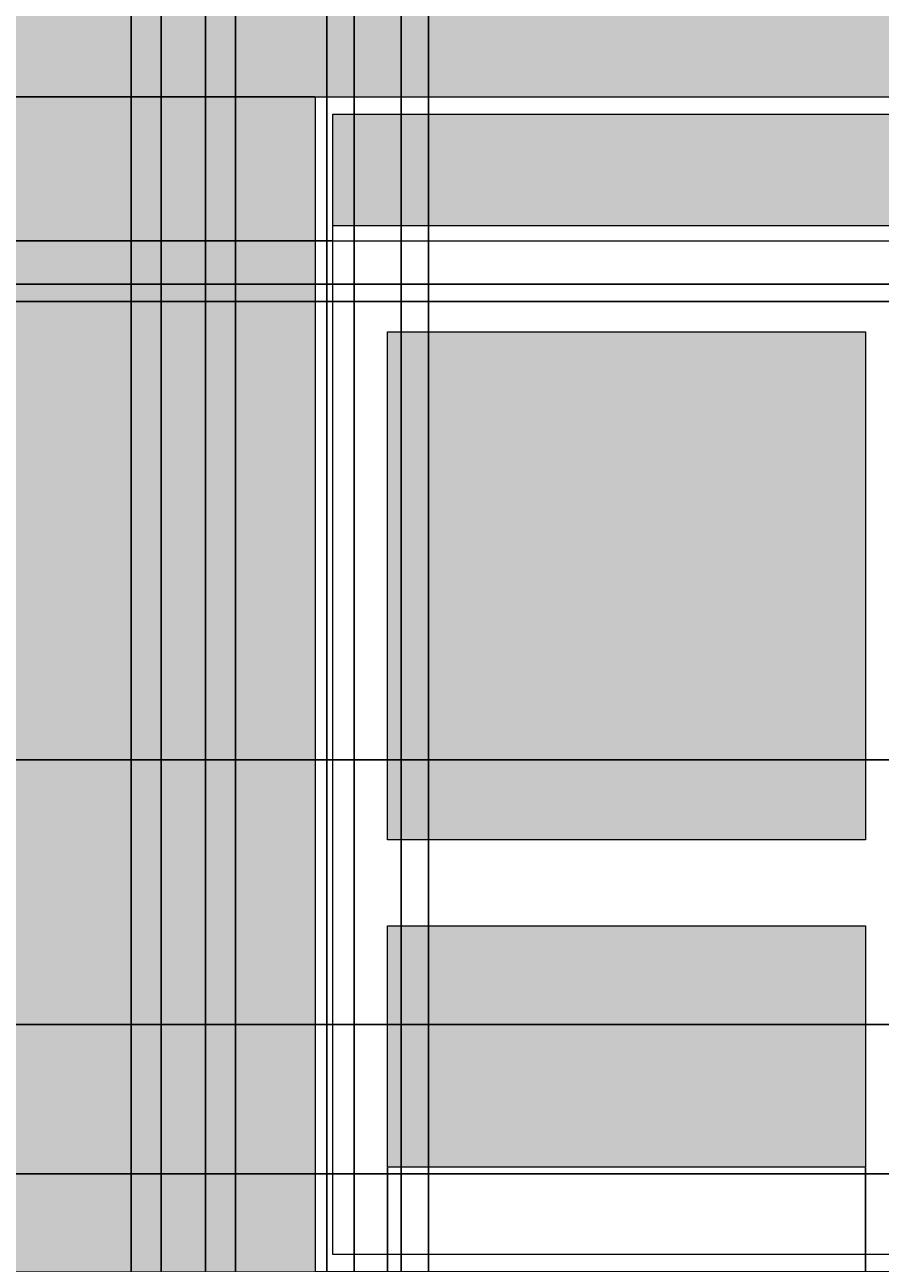
# Model space of a CAD drawing. Units: inches. Extents: x 36 to 594, y 79 to 831.
# Tile 5 of 30: x 221 to 319, y 152 to 294. Entities that reach past the tile are written whole.
import ezdxf

# ---------------------------------------------------------------- set-up
doc = ezdxf.new("R2010")
doc.units = ezdxf.units.IN
doc.header["$MEASUREMENT"] = 0
for name, color, linetype, lineweight in [('A-ANNO-DIMS', 2, 'Continuous', 18), ('A-DOOR', 3, 'Continuous', 18), ('A-ELEV-PATT', 8, 'Continuous', 13)]:
    doc.layers.add(name, color=color, linetype=linetype, lineweight=lineweight)
doc.styles.get("Standard").update_dxf_attribs({"font": 'arial.ttf'})
doc.dimstyles.get("Standard").update_dxf_attribs({"dimtxt": 0.8125, "dimasz": 0.18, "dimexe": 0.18, "dimexo": 0.0625, "dimgap": 0.09, "dimtad": 0, "dimtih": 1, "dimtoh": 1, "dimdec": 4, "dimzin": 0, "dimdsep": 46, "dimlunit": 4, "dimtxsty": 'Standard', "dimcen": 0.09, "dimadec": 0, "dimazin": 0, "dimtfac": 1, "dimtdec": 4, "dimtofl": 0, "dimtmove": 0, "dimatfit": 3, "dimfxl": 1, "dimtolj": 1, "dimtzin": 0, "dimarcsym": 0})

# ---------------------------------------------------------------- blocks, each defined once
blk = doc.blocks.new('*D28')
at = {"layer": 'A-ANNO-DIMS', "color": 0, "lineweight": -2, "transparency": 16777216}
for p, q in [((269.3, 796.05), (37.49, 796.05)), ((37.67, 795.87), (37.67, 455.63)), ((37.67, 114.39), (37.67, 454.62)), ((94.8, 114.21), (37.49, 114.21))]:
    blk.add_line(p, q, dxfattribs=at)
at = {"layer": 'A-ANNO-DIMS', "color": 0, "transparency": 16777216}
for points in [[(37.64, 795.87), (37.7, 795.87), (37.67, 796.05)], [(37.64, 114.39), (37.7, 114.39), (37.67, 114.21)]]:
    blk.add_solid(points, dxfattribs=at)
at = {"layer": 'Defpoints', "color": 0, "transparency": 16777216}
for p in [(37.67, 796.05), (269.36, 796.05), (94.87, 114.21)]:
    blk.add_point(p, dxfattribs=at)
at = {"layer": 'A-ANNO-DIMS', "color": 0, "transparency": 16777216, "insert": (37.67, 455.13), "char_height": 0.812, "attachment_point": 5}
blk.add_mtext('\\A1;681.8', dxfattribs=at)
blk = doc.blocks.new('*D74')
at = {"layer": 'A-ANNO-DIMS', "color": 0, "lineweight": -2, "transparency": 16777216}
for p, q in [((217.09, 179.42), (592.85, 179.42)), ((592.67, 179.24), (592.67, 171.32)), ((592.67, 162.39), (592.67, 170.31)), ((217.09, 162.21), (592.85, 162.21))]:
    blk.add_line(p, q, dxfattribs=at)
at = {"layer": 'A-ANNO-DIMS', "color": 0, "transparency": 16777216}
for points in [[(592.64, 179.24), (592.7, 179.24), (592.67, 179.42)], [(592.64, 162.39), (592.7, 162.39), (592.67, 162.21)]]:
    blk.add_solid(points, dxfattribs=at)
at = {"layer": 'Defpoints', "color": 0, "transparency": 16777216}
for p in [(217.03, 179.42), (592.67, 179.42), (217.03, 162.21)]:
    blk.add_point(p, dxfattribs=at)
at = {"layer": 'A-ANNO-DIMS', "color": 0, "transparency": 16777216, "insert": (592.67, 170.82), "char_height": 0.812, "attachment_point": 5}
blk.add_mtext('\\A1;17.207', dxfattribs=at)
blk = doc.blocks.new('*D75')
at = {"layer": 'A-ANNO-DIMS', "color": 0, "lineweight": -2, "transparency": 16777216}
for p, q in [((215.09, 262.62), (592.85, 262.62)), ((592.67, 262.44), (592.67, 221.53)), ((592.67, 179.6), (592.67, 220.52)), ((217.09, 179.42), (592.85, 179.42))]:
    blk.add_line(p, q, dxfattribs=at)
at = {"layer": 'A-ANNO-DIMS', "color": 0, "transparency": 16777216}
for points in [[(592.64, 262.44), (592.7, 262.44), (592.67, 262.62)], [(592.64, 179.6), (592.7, 179.6), (592.67, 179.42)]]:
    blk.add_solid(points, dxfattribs=at)
at = {"layer": 'Defpoints', "color": 0, "transparency": 16777216}
for p in [(215.03, 262.62), (592.67, 262.62), (217.03, 179.42)]:
    blk.add_point(p, dxfattribs=at)
at = {"layer": 'A-ANNO-DIMS', "color": 0, "transparency": 16777216, "insert": (592.67, 221.02), "char_height": 0.812, "attachment_point": 5}
blk.add_mtext('\\A1;83.2', dxfattribs=at)
blk = doc.blocks.new('*D76')
at = {"layer": 'A-ANNO-DIMS', "color": 0, "lineweight": -2, "transparency": 16777216}
for p, q in [((217.09, 264.62), (592.85, 264.62)), ((592.67, 264.44), (592.67, 264.12)), ((215.09, 262.62), (592.85, 262.62)), ((592.67, 262.8), (592.67, 263.12))]:
    blk.add_line(p, q, dxfattribs=at)
at = {"layer": 'A-ANNO-DIMS', "color": 0, "transparency": 16777216}
for points in [[(592.64, 264.44), (592.7, 264.44), (592.67, 264.62)], [(592.64, 262.8), (592.7, 262.8), (592.67, 262.62)]]:
    blk.add_solid(points, dxfattribs=at)
at = {"layer": 'Defpoints', "color": 0, "transparency": 16777216}
for p in [(217.03, 264.62), (592.67, 264.62), (215.03, 262.62)]:
    blk.add_point(p, dxfattribs=at)
at = {"layer": 'A-ANNO-DIMS', "color": 0, "transparency": 16777216, "insert": (592.67, 263.62), "char_height": 0.812, "attachment_point": 5}
blk.add_mtext('\\A1;2', dxfattribs=at)
blk = doc.blocks.new('*D77')
at = {"layer": 'A-ANNO-DIMS', "color": 0, "lineweight": -2, "transparency": 16777216}
for p, q in [((151.64, 209.88), (592.85, 209.88)), ((592.67, 209.7), (592.67, 186.55)), ((592.67, 162.39), (592.67, 185.54)), ((156.47, 162.21), (592.85, 162.21))]:
    blk.add_line(p, q, dxfattribs=at)
at = {"layer": 'A-ANNO-DIMS', "color": 0, "transparency": 16777216}
for points in [[(592.64, 209.7), (592.7, 209.7), (592.67, 209.88)], [(592.64, 162.39), (592.7, 162.39), (592.67, 162.21)]]:
    blk.add_solid(points, dxfattribs=at)
at = {"layer": 'Defpoints', "color": 0, "transparency": 16777216}
for p in [(151.58, 209.88), (156.41, 162.21), (592.67, 162.21)]:
    blk.add_point(p, dxfattribs=at)
at = {"layer": 'A-ANNO-DIMS', "color": 0, "transparency": 16777216, "insert": (592.67, 186.05), "char_height": 0.812, "attachment_point": 5}
blk.add_mtext('\\A1;47.67', dxfattribs=at)
blk = doc.blocks.new('*D78')
at = {"layer": 'A-ANNO-DIMS', "color": 0, "lineweight": -2, "transparency": 16777216}
for p, q in [((262.32, 162.93), (262.32, 79.53)), ((254.03, 150.87), (254.03, 79.53)), ((254.21, 79.71), (256.71, 79.71)), ((262.14, 79.71), (259.64, 79.71))]:
    blk.add_line(p, q, dxfattribs=at)
at = {"layer": 'A-ANNO-DIMS', "color": 0, "transparency": 16777216}
for points in [[(254.21, 79.74), (254.21, 79.68), (254.03, 79.71)], [(262.14, 79.74), (262.14, 79.68), (262.32, 79.71)]]:
    blk.add_solid(points, dxfattribs=at)
at = {"layer": 'Defpoints', "color": 0, "transparency": 16777216}
for p in [(262.32, 162.99), (254.03, 150.93), (262.32, 79.71)]:
    blk.add_point(p, dxfattribs=at)
at = {"layer": 'A-ANNO-DIMS', "color": 0, "transparency": 16777216, "insert": (258.17, 79.71), "char_height": 0.812, "attachment_point": 5}
blk.add_mtext('\\A1;8.288', dxfattribs=at)
blk = doc.blocks.new('*D79')
at = {"layer": 'A-ANNO-DIMS', "color": 0, "lineweight": -2, "transparency": 16777216}
for p, q in [((262.32, 162.93), (262.32, 79.53)), ((317.35, 162.93), (317.35, 79.53)), ((262.5, 79.71), (288.38, 79.71)), ((317.17, 79.71), (291.29, 79.71))]:
    blk.add_line(p, q, dxfattribs=at)
at = {"layer": 'A-ANNO-DIMS', "color": 0, "transparency": 16777216}
for points in [[(262.5, 79.74), (262.5, 79.68), (262.32, 79.71)], [(317.17, 79.74), (317.17, 79.68), (317.35, 79.71)]]:
    blk.add_solid(points, dxfattribs=at)
at = {"layer": 'Defpoints', "color": 0, "transparency": 16777216}
for p in [(262.32, 162.99), (317.35, 162.99), (317.35, 79.71)]:
    blk.add_point(p, dxfattribs=at)
at = {"layer": 'A-ANNO-DIMS', "color": 0, "transparency": 16777216, "insert": (289.84, 79.71), "char_height": 0.812, "attachment_point": 5}
blk.add_mtext('\\A1;55.04', dxfattribs=at)
blk = doc.blocks.new('*D80')
at = {"layer": 'A-ANNO-DIMS', "color": 0, "lineweight": -2, "transparency": 16777216}
for p, q in [((317.35, 162.93), (317.35, 79.53)), ((327.79, 152.87), (327.79, 79.53)), ((317.53, 79.71), (320.83, 79.71)), ((327.61, 79.71), (324.31, 79.71))]:
    blk.add_line(p, q, dxfattribs=at)
at = {"layer": 'A-ANNO-DIMS', "color": 0, "transparency": 16777216}
for points in [[(317.53, 79.74), (317.53, 79.68), (317.35, 79.71)], [(327.61, 79.74), (327.61, 79.68), (327.79, 79.71)]]:
    blk.add_solid(points, dxfattribs=at)
at = {"layer": 'Defpoints', "color": 0, "transparency": 16777216}
for p in [(317.35, 162.99), (327.79, 152.93), (327.79, 79.71)]:
    blk.add_point(p, dxfattribs=at)
at = {"layer": 'A-ANNO-DIMS', "color": 0, "transparency": 16777216, "insert": (322.57, 79.71), "char_height": 0.812, "attachment_point": 5}
blk.add_mtext('\\A1;10.436', dxfattribs=at)
blk = doc.blocks.new('*D90')
at = {"layer": 'A-ANNO-DIMS', "color": 0, "lineweight": -2, "transparency": 16777216}
for p, q in [((255.97, 269.61), (37.49, 269.61)), ((37.67, 269.43), (37.67, 210.78)), ((37.67, 151.11), (37.67, 209.77)), ((253.97, 150.93), (37.49, 150.93))]:
    blk.add_line(p, q, dxfattribs=at)
at = {"layer": 'A-ANNO-DIMS', "color": 0, "transparency": 16777216}
for points in [[(37.64, 269.43), (37.7, 269.43), (37.67, 269.61)], [(37.64, 151.11), (37.7, 151.11), (37.67, 150.93)]]:
    blk.add_solid(points, dxfattribs=at)
at = {"layer": 'Defpoints', "color": 0, "transparency": 16777216}
for p in [(37.67, 269.61), (256.03, 269.61), (254.03, 150.93)]:
    blk.add_point(p, dxfattribs=at)
at = {"layer": 'A-ANNO-DIMS', "color": 0, "transparency": 16777216, "insert": (37.67, 210.27), "char_height": 0.812, "attachment_point": 5}
blk.add_mtext('\\A1;118.67', dxfattribs=at)
blk = doc.blocks.new('*D91')
at = {"layer": 'A-ANNO-DIMS', "color": 0, "lineweight": -2, "transparency": 16777216}
for p, q in [((253.97, 286.18), (37.49, 286.18)), ((37.67, 286), (37.67, 278.4)), ((37.67, 269.79), (37.67, 277.39)), ((255.97, 269.61), (37.49, 269.61))]:
    blk.add_line(p, q, dxfattribs=at)
at = {"layer": 'A-ANNO-DIMS', "color": 0, "transparency": 16777216}
for points in [[(37.64, 286), (37.7, 286), (37.67, 286.18)], [(37.64, 269.79), (37.7, 269.79), (37.67, 269.61)]]:
    blk.add_solid(points, dxfattribs=at)
at = {"layer": 'Defpoints', "color": 0, "transparency": 16777216}
for p in [(37.67, 286.18), (254.03, 286.18), (256.03, 269.61)]:
    blk.add_point(p, dxfattribs=at)
at = {"layer": 'A-ANNO-DIMS', "color": 0, "transparency": 16777216, "insert": (37.67, 277.89), "char_height": 0.812, "attachment_point": 5}
blk.add_mtext('\\A1;16.572', dxfattribs=at)
blk = doc.blocks.new('*D96')
at = {"layer": 'A-ANNO-DIMS', "color": 0, "lineweight": -2, "transparency": 16777216}
for p, q in [((236.29, 484.36), (236.29, 79.53)), ((232.82, 475.35), (232.82, 79.53)), ((233, 79.71), (233.41, 79.71)), ((236.11, 79.71), (235.7, 79.71))]:
    blk.add_line(p, q, dxfattribs=at)
at = {"layer": 'A-ANNO-DIMS', "color": 0, "transparency": 16777216}
for points in [[(233, 79.74), (233, 79.68), (232.82, 79.71)], [(236.11, 79.74), (236.11, 79.68), (236.29, 79.71)]]:
    blk.add_solid(points, dxfattribs=at)
at = {"layer": 'Defpoints', "color": 0, "transparency": 16777216}
for p in [(236.29, 484.42), (232.82, 475.41), (236.29, 79.71)]:
    blk.add_point(p, dxfattribs=at)
at = {"layer": 'A-ANNO-DIMS', "color": 0, "transparency": 16777216, "insert": (234.56, 79.71), "char_height": 0.812, "attachment_point": 5}
blk.add_mtext('\\A1;3.47', dxfattribs=at)
blk = doc.blocks.new('*D97')
at = {"layer": 'A-ANNO-DIMS', "color": 0, "lineweight": -2, "transparency": 16777216}
for p, q in [((236.29, 484.36), (236.29, 79.53)), ((255.36, 484.36), (255.36, 79.53)), ((236.47, 79.71), (244.09, 79.71)), ((255.18, 79.71), (247.56, 79.71))]:
    blk.add_line(p, q, dxfattribs=at)
at = {"layer": 'A-ANNO-DIMS', "color": 0, "transparency": 16777216}
for points in [[(236.47, 79.74), (236.47, 79.68), (236.29, 79.71)], [(255.18, 79.74), (255.18, 79.68), (255.36, 79.71)]]:
    blk.add_solid(points, dxfattribs=at)
at = {"layer": 'Defpoints', "color": 0, "transparency": 16777216}
for p in [(236.29, 484.42), (255.36, 484.42), (255.36, 79.71)]:
    blk.add_point(p, dxfattribs=at)
at = {"layer": 'A-ANNO-DIMS', "color": 0, "transparency": 16777216, "insert": (245.82, 79.71), "char_height": 0.812, "attachment_point": 5}
blk.add_mtext('\\A1;19.064', dxfattribs=at)
blk = doc.blocks.new('*D98')
at = {"layer": 'A-ANNO-DIMS', "color": 0, "lineweight": -2, "transparency": 16777216}
for p, q in [((255.36, 484.36), (255.36, 79.53)), ((258.51, 475.35), (258.51, 79.53)), ((255.54, 79.71), (255.78, 79.71)), ((258.33, 79.71), (258.08, 79.71))]:
    blk.add_line(p, q, dxfattribs=at)
at = {"layer": 'A-ANNO-DIMS', "color": 0, "transparency": 16777216}
for points in [[(255.54, 79.74), (255.54, 79.68), (255.36, 79.71)], [(258.33, 79.74), (258.33, 79.68), (258.51, 79.71)]]:
    blk.add_solid(points, dxfattribs=at)
at = {"layer": 'Defpoints', "color": 0, "transparency": 16777216}
for p in [(255.36, 484.42), (258.51, 475.41), (258.51, 79.71)]:
    blk.add_point(p, dxfattribs=at)
at = {"layer": 'A-ANNO-DIMS', "color": 0, "transparency": 16777216, "insert": (256.93, 79.71), "char_height": 0.812, "attachment_point": 5}
blk.add_mtext('\\A1;3.15', dxfattribs=at)
blk = doc.blocks.new('*D108')
at = {"layer": 'A-ANNO-DIMS', "color": 0, "lineweight": -2, "transparency": 16777216}
for p, q in [((244.82, 364.03), (244.82, 79.53)), ((241.36, 355.02), (241.36, 79.53)), ((241.54, 79.71), (241.95, 79.71)), ((244.64, 79.71), (244.24, 79.71))]:
    blk.add_line(p, q, dxfattribs=at)
at = {"layer": 'A-ANNO-DIMS', "color": 0, "transparency": 16777216}
for points in [[(241.54, 79.74), (241.54, 79.68), (241.36, 79.71)], [(244.64, 79.74), (244.64, 79.68), (244.82, 79.71)]]:
    blk.add_solid(points, dxfattribs=at)
at = {"layer": 'Defpoints', "color": 0, "transparency": 16777216}
for p in [(244.82, 364.09), (241.36, 355.08), (244.82, 79.71)]:
    blk.add_point(p, dxfattribs=at)
at = {"layer": 'A-ANNO-DIMS', "color": 0, "transparency": 16777216, "insert": (243.09, 79.71), "char_height": 0.812, "attachment_point": 5}
blk.add_mtext('\\A1;3.47', dxfattribs=at)
blk = doc.blocks.new('*D109')
at = {"layer": 'A-ANNO-DIMS', "color": 0, "lineweight": -2, "transparency": 16777216}
for p, q in [((244.82, 364.03), (244.82, 79.53)), ((263.89, 364.03), (263.89, 79.53)), ((245, 79.71), (252.62, 79.71)), ((263.71, 79.71), (256.09, 79.71))]:
    blk.add_line(p, q, dxfattribs=at)
at = {"layer": 'A-ANNO-DIMS', "color": 0, "transparency": 16777216}
for points in [[(245, 79.74), (245, 79.68), (244.82, 79.71)], [(263.71, 79.74), (263.71, 79.68), (263.89, 79.71)]]:
    blk.add_solid(points, dxfattribs=at)
at = {"layer": 'Defpoints', "color": 0, "transparency": 16777216}
for p in [(244.82, 364.09), (263.89, 364.09), (263.89, 79.71)]:
    blk.add_point(p, dxfattribs=at)
at = {"layer": 'A-ANNO-DIMS', "color": 0, "transparency": 16777216, "insert": (254.36, 79.71), "char_height": 0.812, "attachment_point": 5}
blk.add_mtext('\\A1;19.064', dxfattribs=at)
blk = doc.blocks.new('*D110')
at = {"layer": 'A-ANNO-DIMS', "color": 0, "lineweight": -2, "transparency": 16777216}
for p, q in [((263.89, 364.03), (263.89, 79.53)), ((267.04, 355.02), (267.04, 79.53)), ((264.07, 79.71), (264.32, 79.71)), ((266.86, 79.71), (266.61, 79.71))]:
    blk.add_line(p, q, dxfattribs=at)
at = {"layer": 'A-ANNO-DIMS', "color": 0, "transparency": 16777216}
for points in [[(264.07, 79.74), (264.07, 79.68), (263.89, 79.71)], [(266.86, 79.74), (266.86, 79.68), (267.04, 79.71)]]:
    blk.add_solid(points, dxfattribs=at)
at = {"layer": 'Defpoints', "color": 0, "transparency": 16777216}
for p in [(263.89, 364.09), (267.04, 355.08), (267.04, 79.71)]:
    blk.add_point(p, dxfattribs=at)
at = {"layer": 'A-ANNO-DIMS', "color": 0, "transparency": 16777216, "insert": (265.46, 79.71), "char_height": 0.812, "attachment_point": 5}
blk.add_mtext('\\A1;3.15', dxfattribs=at)

msp = doc.modelspace()

# ---------------------------------------------------------------- hatches: boundary and pattern name
at = {"layer": 'A-ELEV-PATT'}
h = msp.add_hatch(color=256, dxfattribs=at)
h.dxf.hatch_style = 1
h.paths.add_polyline_path([(398.0873, 796.0465), (269.3592, 796.0465), (269.3592, 770.1455), (397.8159, 770.1455)])
h.paths.add_polyline_path([(397.7518, 764.0341), (269.3592, 764.0341), (269.3592, 630.0394), (341.8367, 630.0394), (341.8367, 720.595), (335.0881, 728.3699), (329.982, 735.3373), (345.3661, 727.7743), (397.1052, 702.3389)])
h.paths.add_polyline_path([(341.8367, 594.2124), (201.4189, 594.2124), (201.4189, 475.4136), (232.8216, 475.4136), (232.8216, 524.6037), (341.8367, 524.6037)])
h.paths.add_polyline_path([(177.525, 594.2124), (118.7598, 594.2124), (118.7598, 450.2124), (177.525, 450.2124)])
h.paths.add_polyline_path([(424.4958, 594.2124), (365.7306, 594.2124), (365.7306, 450.2124), (424.4958, 450.2124)])
h.paths.add_polyline_path([(241.3553, 404.2737), (355.8569, 404.2737), (355.8569, 355.0836), (424.5492, 355.0836), (424.5492, 425.7333), (118.7598, 426.2844), (118.7598, 355.0836), (241.3553, 355.0836)])
h.paths.add_polyline_path([(448.3898, 306.2124), (217.0273, 306.2124), (217.0273, 142.2124), (254.0293, 142.2124), (254.0293, 150.9347), (254.0293, 286.1802), (401.5491, 286.1802), (401.5491, 150.9347), (401.5491, 142.2124), (448.3898, 142.2124)])
h.paths.add_polyline_path([(448.3898, 142.2124), (401.5491, 142.2124), (217.0273, 142.2124), (217.0273, 114.2124), (448.3898, 114.2124)])
h.paths.add_polyline_path([(217.0273, 306.2124), (174.7353, 306.2124), (94.8658, 306.2124), (94.8658, 162.2124), (103.3368, 162.2124), (103.3368, 264.6224), (103.3368, 286.1802), (217.0273, 286.1802)])
h = msp.add_hatch(color=256, dxfattribs=at)
h.dxf.hatch_style = 1
h.set_gradient(color1=(0, 255, 255), color2=(16, 86, 137))
h.paths.add_polyline_path([(341.8367, 524.6037), (260.5056, 524.6037), (260.5056, 513.1224), (341.8367, 513.1224)])
h.paths.add_polyline_path([(341.8367, 511.1224), (260.5056, 511.1224), (260.5056, 475.4136), (341.8367, 475.4136)])
h.paths.add_polyline_path([(258.5056, 524.6037), (232.8216, 524.6037), (232.8216, 513.1224), (258.5056, 513.1224)])
h.paths.add_polyline_path([(355.8569, 404.2737), (269.0393, 404.2737), (269.0393, 392.7924), (355.8569, 392.7924)])
h.paths.add_polyline_path([(267.0393, 404.2737), (241.3553, 404.2737), (241.3553, 392.7924), (267.0393, 392.7924)])
h.paths.add_polyline_path([(355.8569, 390.7924), (269.0393, 390.7924), (269.0393, 355.0836), (355.8569, 355.0836)])
h.paths.add_polyline_path([(399.5491, 284.1802), (256.0293, 284.1802), (256.0293, 271.378), (399.5491, 271.378)])
h.paths.add_polyline_path([(317.3533, 259.1243), (262.3169, 259.1243), (262.3169, 200.6645), (317.3533, 200.6645)])
h.paths.add_polyline_path([(390.386, 259.1243), (335.3496, 259.1243), (335.3496, 200.6645), (390.386, 200.6645)])
h.paths.add_polyline_path([(390.386, 190.7697), (335.3496, 190.7697), (335.3496, 162.9881), (390.386, 162.9881)])
h.paths.add_polyline_path([(317.3533, 190.7697), (262.3169, 190.7697), (262.3169, 162.9881), (317.3533, 162.9881)])
h.paths.add_polyline_path([(215.0273, 262.6224), (158.4069, 262.6224), (158.4069, 181.4195), (215.0273, 181.4195)])
h.paths.add_polyline_path([(215.0273, 284.1802), (105.3368, 284.1802), (105.3368, 266.6224), (215.0273, 266.6224)])

# ---------------------------------------------------------------- linework, layer by layer
at = {"layer": 'A-DOOR'}
msp.add_line((256.0293, 271.378), (399.5491, 271.378), dxfattribs=at)
for points in [[(254.0293, 286.1802), (401.5491, 286.1802), (401.5491, 150.9347), (254.0293, 150.9347)], [(256.0293, 284.1802), (399.5491, 284.1802), (399.5491, 152.9347), (256.0293, 152.9347)], [(256.0293, 269.6084), (327.7892, 269.6084), (327.7892, 152.9347), (256.0293, 152.9347)], [(262.3169, 259.1243), (317.3533, 259.1243), (317.3533, 200.6645), (262.3169, 200.6645)], [(262.3169, 190.7697), (317.3533, 190.7697), (317.3533, 162.9881), (262.3169, 162.9881)]]:
    msp.add_lwpolyline(points, close=True, dxfattribs=at)

# ---------------------------------------------------------------- dimensions: what is measured, and where the dimension line sits
at = {"layer": 'A-ANNO-DIMS'}
for base, p1, p2, override, picture, middle in [((37.6733, 796.0465), (94.8658, 114.2124), (269.3592, 796.0465), {"dimdec": 1, "dimlfac": 1, "dimrnd": 0, "dimzin": 0, "dimdsep": 46, "dimlunit": 2}, '*D28', (37.6733, 455.1294)), ((37.6733, 286.1802), (256.0293, 269.6084), (254.0293, 286.1802), {"dimdec": 3, "dimlfac": 1, "dimrnd": 0, "dimzin": 0, "dimdsep": 46, "dimlunit": 2}, '*D91', (37.6733, 277.8943)), ((37.6733, 269.6084), (254.0293, 150.9347), (256.0293, 269.6084), {"dimdec": 2, "dimlfac": 1, "dimrnd": 0, "dimzin": 0, "dimdsep": 46, "dimlunit": 2}, '*D90', (37.6733, 210.2716)), ((592.6689, 264.6224), (215.0273, 262.6224), (217.0273, 264.6224), {"dimdec": 0, "dimlfac": 1, "dimrnd": 0, "dimzin": 0, "dimdsep": 46, "dimlunit": 2}, '*D76', (592.6689, 263.6224)), ((592.6689, 262.6224), (217.0273, 179.4195), (215.0273, 262.6224), {"dimdec": 1, "dimlfac": 1, "dimrnd": 0, "dimzin": 0, "dimdsep": 46, "dimlunit": 2}, '*D75', (592.6689, 221.021)), ((592.6689, 162.2124), (151.5799, 209.8823), (156.4069, 162.2124), {"dimdec": 2, "dimlfac": 1, "dimrnd": 0, "dimzin": 0, "dimdsep": 46, "dimlunit": 2}, '*D77', (592.6689, 186.0473)), ((592.6689, 179.4195), (217.0273, 162.2124), (217.0273, 179.4195), {"dimdec": 3, "dimlfac": 1, "dimrnd": 0, "dimzin": 0, "dimdsep": 46, "dimlunit": 2}, '*D74', (592.6689, 170.8159))]:
    dim = msp.add_linear_dim(base=base, p1=p1, p2=p2, angle=90, dimstyle='Standard', override=override, dxfattribs=at)
    dim.commit()
    dim.dimension.update_dxf_attribs({"geometry": picture, "text_midpoint": middle})
for base, p1, p2, override, picture, middle in [((236.2911, 79.7124), (232.8216, 475.4136), (236.2911, 484.4187), {"dimdec": 2, "dimlfac": 1, "dimrnd": 0, "dimzin": 0, "dimdsep": 46, "dimlunit": 2}, '*D96', (234.5563, 79.7124)), ((255.3555, 79.7124), (236.2911, 484.4187), (255.3555, 484.4187), {"dimdec": 3, "dimlfac": 1, "dimrnd": 0, "dimzin": 0, "dimdsep": 46, "dimlunit": 2}, '*D97', (245.8233, 79.7124)), ((258.5056, 79.7124), (255.3555, 484.4187), (258.5056, 475.4136), {"dimdec": 2, "dimlfac": 1, "dimrnd": 0, "dimzin": 0, "dimdsep": 46, "dimlunit": 2}, '*D98', (256.9305, 79.7124)), ((244.8248, 79.7124), (241.3553, 355.0836), (244.8248, 364.0887), {"dimdec": 2, "dimlfac": 1, "dimrnd": 0, "dimzin": 0, "dimdsep": 46, "dimlunit": 2}, '*D108', (243.09, 79.7124)), ((263.8892, 79.7124), (244.8248, 364.0887), (263.8892, 364.0887), {"dimdec": 3, "dimlfac": 1, "dimrnd": 0, "dimzin": 0, "dimdsep": 46, "dimlunit": 2}, '*D109', (254.357, 79.7124)), ((267.0393, 79.7124), (263.8892, 364.0887), (267.0393, 355.0836), {"dimdec": 2, "dimlfac": 1, "dimrnd": 0, "dimzin": 0, "dimdsep": 46, "dimlunit": 2}, '*D110', (265.4643, 79.7124)), ((262.3169, 79.7124), (254.0293, 150.9347), (262.3169, 162.9881), {"dimdec": 3, "dimlfac": 1, "dimrnd": 0, "dimzin": 0, "dimdsep": 46, "dimlunit": 2}, '*D78', (258.1731, 79.7124)), ((317.3533, 79.7124), (262.3169, 162.9881), (317.3533, 162.9881), {"dimdec": 2, "dimlfac": 1, "dimrnd": 0, "dimzin": 0, "dimdsep": 46, "dimlunit": 2}, '*D79', (289.8351, 79.7124)), ((327.7892, 79.7124), (317.3533, 162.9881), (327.7892, 152.9347), {"dimdec": 3, "dimlfac": 1, "dimrnd": 0, "dimzin": 0, "dimdsep": 46, "dimlunit": 2}, '*D80', (322.5712, 79.7124))]:
    dim = msp.add_linear_dim(base=base, p1=p1, p2=p2, dimstyle='Standard', override=override, dxfattribs=at)
    dim.commit()
    dim.dimension.update_dxf_attribs({"geometry": picture, "text_midpoint": middle})

doc.saveas('drawing.dxf')
